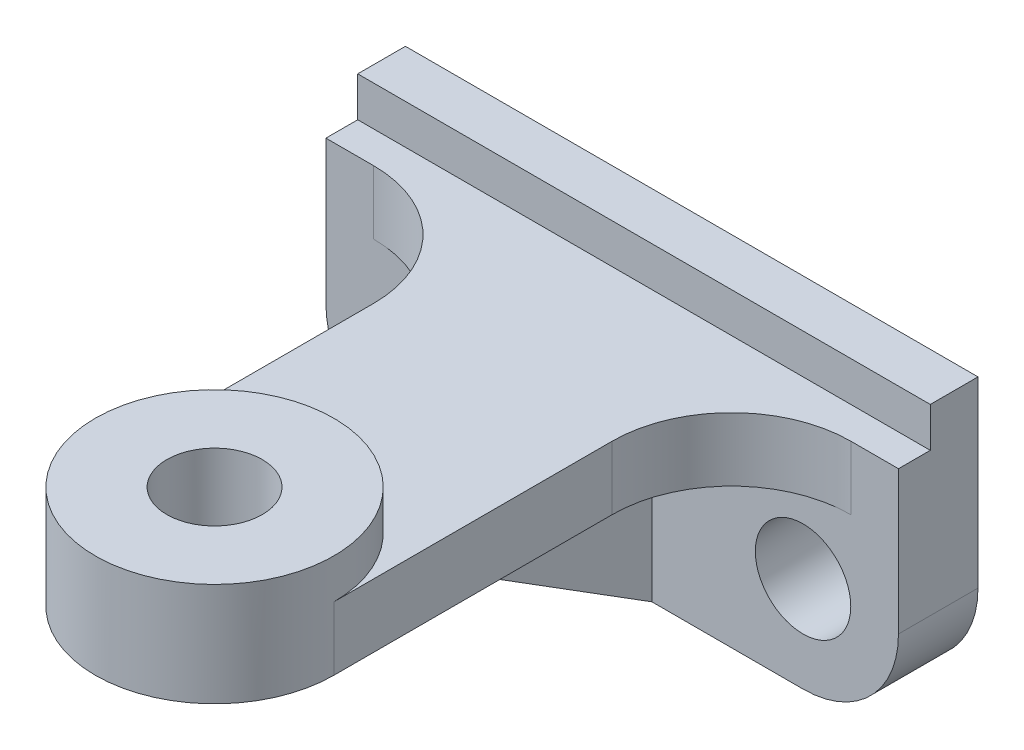
ISO-10303-21;
HEADER;
FILE_DESCRIPTION(('STEP AP214'),'2;1');
FILE_NAME('part.step','',(''),(''),'','','');
FILE_SCHEMA(('AUTOMOTIVE_DESIGN { 1 0 10303 214 1 1 1 1 }'));
ENDSEC;
DATA;
#1=APPLICATION_CONTEXT('core data for automotive mechanical design processes');
#2=APPLICATION_PROTOCOL_DEFINITION('international standard','automotive_design',2000,#1);
#3=PRODUCT_CONTEXT('',#1,'mechanical');
#4=PRODUCT('Part','Part','',(#3));
#5=PRODUCT_RELATED_PRODUCT_CATEGORY('part','',(#4));
#6=PRODUCT_DEFINITION_FORMATION('','',#4);
#7=PRODUCT_DEFINITION_CONTEXT('part definition',#1,'design');
#8=PRODUCT_DEFINITION('design','',#6,#7);
#9=PRODUCT_DEFINITION_SHAPE('','',#8);
#10=(LENGTH_UNIT() NAMED_UNIT(*) SI_UNIT(.MILLI.,.METRE.));
#11=(NAMED_UNIT(*) PLANE_ANGLE_UNIT() SI_UNIT($,.RADIAN.));
#12=(NAMED_UNIT(*) SI_UNIT($,.STERADIAN.) SOLID_ANGLE_UNIT());
#13=UNCERTAINTY_MEASURE_WITH_UNIT(LENGTH_MEASURE(1.E-05),#10,'distance_accuracy_value','');
#14=(GEOMETRIC_REPRESENTATION_CONTEXT(3) GLOBAL_UNCERTAINTY_ASSIGNED_CONTEXT((#13)) GLOBAL_UNIT_ASSIGNED_CONTEXT((#10,
#11,#12)) REPRESENTATION_CONTEXT('',''));
#15=CARTESIAN_POINT('',(0.,0.,0.));
#16=DIRECTION('',(0.,0.,1.));
#17=DIRECTION('',(1.,0.,0.));
#18=AXIS2_PLACEMENT_3D('',#15,#16,#17);
#19=CARTESIAN_POINT('',(72.,-13.,45.0717511200109));
#20=DIRECTION('',(0.,-0.847127010038503,0.531390467418476));
#21=DIRECTION('',(0.,-0.531390467418476,-0.847127010038503));
#22=AXIS2_PLACEMENT_3D('',#19,#20,#21);
#23=PLANE('',#22);
#24=DIRECTION('',(0.,0.531390467418476,0.847127010038503));
#25=VECTOR('',#24,1.);
#26=CARTESIAN_POINT('',(31.,-13.,45.0717511200109));
#27=LINE('',#26,#25);
#28=CARTESIAN_POINT('',(31.,-35.,10.));
#29=VERTEX_POINT('',#28);
#30=CARTESIAN_POINT('',(31.,-13.,45.0717511200109));
#31=VERTEX_POINT('',#30);
#32=EDGE_CURVE('E183',#29,#31,#27,.T.);
#33=ORIENTED_EDGE('',*,*,#32,.F.);
#34=DIRECTION('',(1.,0.,0.));
#35=VECTOR('',#34,1.);
#36=CARTESIAN_POINT('',(0.,-35.,10.));
#37=LINE('',#36,#35);
#38=CARTESIAN_POINT('',(41.,-35.,10.));
#39=VERTEX_POINT('',#38);
#40=EDGE_CURVE('E277',#29,#39,#37,.T.);
#41=ORIENTED_EDGE('',*,*,#40,.T.);
#42=DIRECTION('',(0.,-0.531390467418476,-0.847127010038503));
#43=VECTOR('',#42,1.);
#44=CARTESIAN_POINT('',(41.,-35.,10.));
#45=LINE('',#44,#43);
#46=CARTESIAN_POINT('',(41.,-13.,45.0717511200109));
#47=VERTEX_POINT('',#46);
#48=EDGE_CURVE('E192',#47,#39,#45,.T.);
#49=ORIENTED_EDGE('',*,*,#48,.F.);
#50=DIRECTION('',(-1.,0.,0.));
#51=VECTOR('',#50,1.);
#52=CARTESIAN_POINT('',(72.,-13.,45.0717511200109));
#53=LINE('',#52,#51);
#54=EDGE_CURVE('E180',#47,#31,#53,.T.);
#55=ORIENTED_EDGE('',*,*,#54,.T.);
#56=EDGE_LOOP('',(#33,#41,#49,#55));
#57=FACE_BOUND('',#56,.T.);
#58=ADVANCED_FACE('F50',(#57),#23,.T.);
#59=CARTESIAN_POINT('',(0.,0.,10.));
#60=DIRECTION('',(0.,0.,1.));
#61=DIRECTION('',(1.,0.,0.));
#62=AXIS2_PLACEMENT_3D('',#59,#60,#61);
#63=PLANE('',#62);
#64=DIRECTION('',(0.,-1.,0.));
#65=VECTOR('',#64,1.);
#66=CARTESIAN_POINT('',(66.,-5.,10.));
#67=LINE('',#66,#65);
#68=CARTESIAN_POINT('',(66.,-5.,10.));
#69=VERTEX_POINT('',#68);
#70=CARTESIAN_POINT('',(66.,-13.,10.));
#71=VERTEX_POINT('',#70);
#72=EDGE_CURVE('E212',#69,#71,#67,.T.);
#73=ORIENTED_EDGE('',*,*,#72,.T.);
#74=DIRECTION('',(1.,0.,0.));
#75=VECTOR('',#74,1.);
#76=CARTESIAN_POINT('',(41.,-13.0000000000001,10.));
#77=LINE('',#76,#75);
#78=CARTESIAN_POINT('',(41.,-13.0000000000001,10.));
#79=VERTEX_POINT('',#78);
#80=EDGE_CURVE('E200',#79,#71,#77,.T.);
#81=ORIENTED_EDGE('',*,*,#80,.F.);
#82=DIRECTION('',(0.,1.,0.));
#83=VECTOR('',#82,1.);
#84=CARTESIAN_POINT('',(41.,-13.0000000000001,10.));
#85=LINE('',#84,#83);
#86=EDGE_CURVE('E369',#39,#79,#85,.T.);
#87=ORIENTED_EDGE('',*,*,#86,.F.);
#88=DIRECTION('',(1.,0.,0.));
#89=VECTOR('',#88,1.);
#90=CARTESIAN_POINT('',(41.,-35.,10.));
#91=LINE('',#90,#89);
#92=CARTESIAN_POINT('',(60.,-35.,10.));
#93=VERTEX_POINT('',#92);
#94=EDGE_CURVE('E201',#39,#93,#91,.T.);
#95=ORIENTED_EDGE('',*,*,#94,.T.);
#96=CARTESIAN_POINT('',(60.,-23.,10.));
#97=DIRECTION('',(0.,0.,1.));
#98=DIRECTION('',(1.,0.,0.));
#99=AXIS2_PLACEMENT_3D('',#96,#97,#98);
#100=CIRCLE('',#99,12.);
#101=CARTESIAN_POINT('',(72.,-23.,10.));
#102=VERTEX_POINT('',#101);
#103=EDGE_CURVE('E266',#93,#102,#100,.T.);
#104=ORIENTED_EDGE('',*,*,#103,.T.);
#105=DIRECTION('',(0.,-1.,0.));
#106=VECTOR('',#105,1.);
#107=CARTESIAN_POINT('',(72.,0.,10.));
#108=LINE('',#107,#106);
#109=CARTESIAN_POINT('',(72.,-5.,10.));
#110=VERTEX_POINT('',#109);
#111=EDGE_CURVE('E268',#110,#102,#108,.T.);
#112=ORIENTED_EDGE('',*,*,#111,.F.);
#113=DIRECTION('',(1.,0.,0.));
#114=VECTOR('',#113,1.);
#115=CARTESIAN_POINT('',(0.,-5.00000000000004,10.));
#116=LINE('',#115,#114);
#117=EDGE_CURVE('E310',#69,#110,#116,.T.);
#118=ORIENTED_EDGE('',*,*,#117,.F.);
#119=EDGE_LOOP('',(#73,#81,#87,#95,#104,#112,#118));
#120=FACE_BOUND('',#119,.T.);
#121=CARTESIAN_POINT('',(60.,-23.,10.));
#122=DIRECTION('',(0.,0.,-1.));
#123=DIRECTION('',(-1.,0.,0.));
#124=AXIS2_PLACEMENT_3D('',#121,#122,#123);
#125=CIRCLE('',#124,6.);
#126=CARTESIAN_POINT('',(54.,-23.,10.));
#127=VERTEX_POINT('',#126);
#128=EDGE_CURVE('E194',#127,#127,#125,.F.);
#129=ORIENTED_EDGE('',*,*,#128,.F.);
#130=EDGE_LOOP('',(#129));
#131=FACE_BOUND('',#130,.T.);
#132=ADVANCED_FACE('F316',(#120,#131),#63,.T.);
#133=CARTESIAN_POINT('',(51.,-17.,10.));
#134=DIRECTION('',(1.,0.,0.));
#135=DIRECTION('',(0.,1.,0.));
#136=AXIS2_PLACEMENT_3D('',#133,#134,#135);
#137=PLANE('',#136);
#138=DIRECTION('',(0.,0.,1.));
#139=VECTOR('',#138,1.);
#140=CARTESIAN_POINT('',(51.,-13.,10.));
#141=LINE('',#140,#139);
#142=CARTESIAN_POINT('',(51.,-13.,25.));
#143=VERTEX_POINT('',#142);
#144=CARTESIAN_POINT('',(51.,-13.,60.));
#145=VERTEX_POINT('',#144);
#146=EDGE_CURVE('E235',#143,#145,#141,.T.);
#147=ORIENTED_EDGE('',*,*,#146,.F.);
#148=DIRECTION('',(0.,-1.,0.));
#149=VECTOR('',#148,1.);
#150=CARTESIAN_POINT('',(51.,-5.00000000000001,25.));
#151=LINE('',#150,#149);
#152=CARTESIAN_POINT('',(51.,-5.00000000000001,25.));
#153=VERTEX_POINT('',#152);
#154=EDGE_CURVE('E206',#153,#143,#151,.T.);
#155=ORIENTED_EDGE('',*,*,#154,.F.);
#156=DIRECTION('',(0.,0.,-1.));
#157=VECTOR('',#156,1.);
#158=CARTESIAN_POINT('',(51.,-5.00000000000001,10.));
#159=LINE('',#158,#157);
#160=CARTESIAN_POINT('',(51.,-5.00000000000001,60.));
#161=VERTEX_POINT('',#160);
#162=EDGE_CURVE('E245',#161,#153,#159,.T.);
#163=ORIENTED_EDGE('',*,*,#162,.F.);
#164=DIRECTION('',(0.,1.,0.));
#165=VECTOR('',#164,1.);
#166=CARTESIAN_POINT('',(51.,-17.,60.));
#167=LINE('',#166,#165);
#168=EDGE_CURVE('E248',#145,#161,#167,.T.);
#169=ORIENTED_EDGE('',*,*,#168,.F.);
#170=EDGE_LOOP('',(#147,#155,#163,#169));
#171=FACE_BOUND('',#170,.T.);
#172=ADVANCED_FACE('F366',(#171),#137,.T.);
#173=DIRECTION('',(0.,-1.,0.));
#174=VECTOR('',#173,1.);
#175=CARTESIAN_POINT('',(0.,0.,10.));
#176=LINE('',#175,#174);
#177=CARTESIAN_POINT('',(0.,-5.00000000000002,10.));
#178=VERTEX_POINT('',#177);
#179=CARTESIAN_POINT('',(0.,-23.,10.));
#180=VERTEX_POINT('',#179);
#181=EDGE_CURVE('E275',#178,#180,#176,.T.);
#182=ORIENTED_EDGE('',*,*,#181,.T.);
#183=CARTESIAN_POINT('',(12.,-23.,10.));
#184=DIRECTION('',(0.,0.,1.));
#185=DIRECTION('',(1.,0.,0.));
#186=AXIS2_PLACEMENT_3D('',#183,#184,#185);
#187=CIRCLE('',#186,12.);
#188=CARTESIAN_POINT('',(12.,-35.,10.));
#189=VERTEX_POINT('',#188);
#190=EDGE_CURVE('E274',#180,#189,#187,.T.);
#191=ORIENTED_EDGE('',*,*,#190,.T.);
#192=EDGE_CURVE('E280',#189,#29,#37,.T.);
#193=ORIENTED_EDGE('',*,*,#192,.T.);
#194=DIRECTION('',(0.,-1.,0.));
#195=VECTOR('',#194,1.);
#196=CARTESIAN_POINT('',(31.,-35.,10.));
#197=LINE('',#196,#195);
#198=CARTESIAN_POINT('',(31.,-13.,10.));
#199=VERTEX_POINT('',#198);
#200=EDGE_CURVE('E182',#199,#29,#197,.T.);
#201=ORIENTED_EDGE('',*,*,#200,.F.);
#202=DIRECTION('',(-1.,0.,0.));
#203=VECTOR('',#202,1.);
#204=CARTESIAN_POINT('',(31.,-13.,10.));
#205=LINE('',#204,#203);
#206=CARTESIAN_POINT('',(5.99999999999999,-13.,10.));
#207=VERTEX_POINT('',#206);
#208=EDGE_CURVE('E177',#199,#207,#205,.T.);
#209=ORIENTED_EDGE('',*,*,#208,.T.);
#210=DIRECTION('',(0.,-1.,0.));
#211=VECTOR('',#210,1.);
#212=CARTESIAN_POINT('',(5.99999999999998,-5.00000000000004,10.));
#213=LINE('',#212,#211);
#214=CARTESIAN_POINT('',(5.99999999999998,-5.00000000000004,10.));
#215=VERTEX_POINT('',#214);
#216=EDGE_CURVE('E217',#215,#207,#213,.T.);
#217=ORIENTED_EDGE('',*,*,#216,.F.);
#218=EDGE_CURVE('E57',#178,#215,#116,.T.);
#219=ORIENTED_EDGE('',*,*,#218,.F.);
#220=EDGE_LOOP('',(#182,#191,#193,#201,#209,#217,#219));
#221=FACE_BOUND('',#220,.T.);
#222=CARTESIAN_POINT('',(12.,-23.,10.));
#223=DIRECTION('',(0.,0.,-1.));
#224=DIRECTION('',(-1.,0.,0.));
#225=AXIS2_PLACEMENT_3D('',#222,#223,#224);
#226=CIRCLE('',#225,6.);
#227=CARTESIAN_POINT('',(5.99999999999999,-23.,10.));
#228=VERTEX_POINT('',#227);
#229=EDGE_CURVE('E204',#228,#228,#226,.F.);
#230=ORIENTED_EDGE('',*,*,#229,.F.);
#231=EDGE_LOOP('',(#230));
#232=FACE_BOUND('',#231,.T.);
#233=ADVANCED_FACE('F343',(#221,#232),#63,.T.);
#234=CARTESIAN_POINT('',(36.,-17.,60.));
#235=DIRECTION('',(0.,1.,0.));
#236=DIRECTION('',(-1.,0.,0.));
#237=AXIS2_PLACEMENT_3D('',#234,#235,#236);
#238=CYLINDRICAL_SURFACE('',#237,15.);
#239=CARTESIAN_POINT('',(36.,0.,60.));
#240=DIRECTION('',(0.,1.,0.));
#241=DIRECTION('',(-1.,0.,0.));
#242=AXIS2_PLACEMENT_3D('',#239,#240,#241);
#243=CIRCLE('',#242,15.);
#244=CARTESIAN_POINT('',(21.,0.,60.));
#245=VERTEX_POINT('',#244);
#246=EDGE_CURVE('E237',#245,#245,#243,.T.);
#247=ORIENTED_EDGE('',*,*,#246,.F.);
#248=EDGE_LOOP('',(#247));
#249=FACE_BOUND('',#248,.T.);
#250=DIRECTION('',(0.,1.,0.));
#251=VECTOR('',#250,1.);
#252=CARTESIAN_POINT('',(21.,-17.,60.));
#253=LINE('',#252,#251);
#254=CARTESIAN_POINT('',(21.,-13.,60.));
#255=VERTEX_POINT('',#254);
#256=CARTESIAN_POINT('',(21.,-5.00000000000003,60.));
#257=VERTEX_POINT('',#256);
#258=EDGE_CURVE('E249',#255,#257,#253,.T.);
#259=ORIENTED_EDGE('',*,*,#258,.F.);
#260=CARTESIAN_POINT('',(36.,-13.,60.));
#261=DIRECTION('',(0.,-1.,0.));
#262=DIRECTION('',(1.,0.,0.));
#263=AXIS2_PLACEMENT_3D('',#260,#261,#262);
#264=CIRCLE('',#263,15.);
#265=EDGE_CURVE('E234',#145,#255,#264,.T.);
#266=ORIENTED_EDGE('',*,*,#265,.F.);
#267=ORIENTED_EDGE('',*,*,#168,.T.);
#268=CARTESIAN_POINT('',(36.,-5.00000000000002,60.));
#269=DIRECTION('',(0.,1.,0.));
#270=DIRECTION('',(-1.,0.,0.));
#271=AXIS2_PLACEMENT_3D('',#268,#269,#270);
#272=CIRCLE('',#271,15.);
#273=EDGE_CURVE('E238',#161,#257,#272,.T.);
#274=ORIENTED_EDGE('',*,*,#273,.T.);
#275=EDGE_LOOP('',(#259,#266,#267,#274));
#276=FACE_BOUND('',#275,.T.);
#277=ADVANCED_FACE('F359',(#249,#276),#238,.T.);
#278=CARTESIAN_POINT('',(21.,-17.,60.));
#279=DIRECTION('',(-1.,0.,0.));
#280=DIRECTION('',(0.,-1.,0.));
#281=AXIS2_PLACEMENT_3D('',#278,#279,#280);
#282=PLANE('',#281);
#283=DIRECTION('',(0.,-1.,0.));
#284=VECTOR('',#283,1.);
#285=CARTESIAN_POINT('',(21.,-5.00000000000003,25.));
#286=LINE('',#285,#284);
#287=CARTESIAN_POINT('',(21.,-5.00000000000003,25.));
#288=VERTEX_POINT('',#287);
#289=CARTESIAN_POINT('',(21.,-13.,25.));
#290=VERTEX_POINT('',#289);
#291=EDGE_CURVE('E221',#288,#290,#286,.T.);
#292=ORIENTED_EDGE('',*,*,#291,.T.);
#293=DIRECTION('',(0.,0.,-1.));
#294=VECTOR('',#293,1.);
#295=CARTESIAN_POINT('',(21.,-13.,10.));
#296=LINE('',#295,#294);
#297=EDGE_CURVE('E236',#255,#290,#296,.T.);
#298=ORIENTED_EDGE('',*,*,#297,.F.);
#299=ORIENTED_EDGE('',*,*,#258,.T.);
#300=DIRECTION('',(0.,0.,1.));
#301=VECTOR('',#300,1.);
#302=CARTESIAN_POINT('',(21.,-5.00000000000003,60.));
#303=LINE('',#302,#301);
#304=EDGE_CURVE('E250',#288,#257,#303,.T.);
#305=ORIENTED_EDGE('',*,*,#304,.F.);
#306=EDGE_LOOP('',(#292,#298,#299,#305));
#307=FACE_BOUND('',#306,.T.);
#308=ADVANCED_FACE('F355',(#307),#282,.T.);
#309=CARTESIAN_POINT('',(-78.,-5.00000000000009,6.));
#310=DIRECTION('',(0.,-1.,0.));
#311=DIRECTION('',(1.,0.,0.));
#312=AXIS2_PLACEMENT_3D('',#309,#310,#311);
#313=PLANE('',#312);
#314=CARTESIAN_POINT('',(66.,-5.,25.));
#315=DIRECTION('',(0.,1.,0.));
#316=DIRECTION('',(1.,0.,0.));
#317=AXIS2_PLACEMENT_3D('',#314,#315,#316);
#318=CIRCLE('',#317,15.);
#319=EDGE_CURVE('E207',#69,#153,#318,.T.);
#320=ORIENTED_EDGE('',*,*,#319,.F.);
#321=ORIENTED_EDGE('',*,*,#117,.T.);
#322=DIRECTION('',(0.,0.,-1.));
#323=VECTOR('',#322,1.);
#324=CARTESIAN_POINT('',(72.,-5.,6.));
#325=LINE('',#324,#323);
#326=CARTESIAN_POINT('',(72.,-5.,6.));
#327=VERTEX_POINT('',#326);
#328=EDGE_CURVE('E254',#110,#327,#325,.T.);
#329=ORIENTED_EDGE('',*,*,#328,.T.);
#330=DIRECTION('',(1.,0.,0.));
#331=VECTOR('',#330,1.);
#332=CARTESIAN_POINT('',(-78.,-5.00000000000009,6.));
#333=LINE('',#332,#331);
#334=CARTESIAN_POINT('',(0.,-5.00000000000004,6.));
#335=VERTEX_POINT('',#334);
#336=EDGE_CURVE('E256',#335,#327,#333,.T.);
#337=ORIENTED_EDGE('',*,*,#336,.F.);
#338=DIRECTION('',(0.,0.,-1.));
#339=VECTOR('',#338,1.);
#340=CARTESIAN_POINT('',(0.,-5.00000000000004,10.));
#341=LINE('',#340,#339);
#342=EDGE_CURVE('E72',#178,#335,#341,.T.);
#343=ORIENTED_EDGE('',*,*,#342,.F.);
#344=ORIENTED_EDGE('',*,*,#218,.T.);
#345=CARTESIAN_POINT('',(5.99999999999999,-5.00000000000004,25.));
#346=DIRECTION('',(0.,1.,0.));
#347=DIRECTION('',(-1.,0.,0.));
#348=AXIS2_PLACEMENT_3D('',#345,#346,#347);
#349=CIRCLE('',#348,15.);
#350=EDGE_CURVE('E220',#288,#215,#349,.T.);
#351=ORIENTED_EDGE('',*,*,#350,.F.);
#352=ORIENTED_EDGE('',*,*,#304,.T.);
#353=ORIENTED_EDGE('',*,*,#273,.F.);
#354=ORIENTED_EDGE('',*,*,#162,.T.);
#355=EDGE_LOOP('',(#320,#321,#329,#337,#343,#344,#351,#352,#353,#354));
#356=FACE_BOUND('',#355,.T.);
#357=ADVANCED_FACE('F315',(#356),#313,.F.);
#358=CARTESIAN_POINT('',(60.,-23.,10.));
#359=DIRECTION('',(0.,0.,-1.));
#360=DIRECTION('',(-1.,0.,0.));
#361=AXIS2_PLACEMENT_3D('',#358,#359,#360);
#362=CYLINDRICAL_SURFACE('',#361,12.);
#363=CARTESIAN_POINT('',(60.,-23.,0.));
#364=DIRECTION('',(0.,0.,1.));
#365=DIRECTION('',(1.,0.,0.));
#366=AXIS2_PLACEMENT_3D('',#363,#364,#365);
#367=CIRCLE('',#366,12.);
#368=CARTESIAN_POINT('',(60.,-35.,0.));
#369=VERTEX_POINT('',#368);
#370=CARTESIAN_POINT('',(72.,-23.,0.));
#371=VERTEX_POINT('',#370);
#372=EDGE_CURVE('E264',#369,#371,#367,.T.);
#373=ORIENTED_EDGE('',*,*,#372,.T.);
#374=DIRECTION('',(0.,0.,-1.));
#375=VECTOR('',#374,1.);
#376=CARTESIAN_POINT('',(72.,-23.,10.));
#377=LINE('',#376,#375);
#378=EDGE_CURVE('E304',#102,#371,#377,.T.);
#379=ORIENTED_EDGE('',*,*,#378,.F.);
#380=ORIENTED_EDGE('',*,*,#103,.F.);
#381=DIRECTION('',(0.,0.,-1.));
#382=VECTOR('',#381,1.);
#383=CARTESIAN_POINT('',(60.,-35.,10.));
#384=LINE('',#383,#382);
#385=EDGE_CURVE('E276',#93,#369,#384,.T.);
#386=ORIENTED_EDGE('',*,*,#385,.T.);
#387=EDGE_LOOP('',(#373,#379,#380,#386));
#388=FACE_BOUND('',#387,.T.);
#389=ADVANCED_FACE('F47',(#388),#362,.T.);
#390=CARTESIAN_POINT('',(72.,0.,10.));
#391=DIRECTION('',(1.,0.,0.));
#392=DIRECTION('',(0.,1.,0.));
#393=AXIS2_PLACEMENT_3D('',#390,#391,#392);
#394=PLANE('',#393);
#395=ORIENTED_EDGE('',*,*,#111,.T.);
#396=ORIENTED_EDGE('',*,*,#378,.T.);
#397=DIRECTION('',(0.,-1.,0.));
#398=VECTOR('',#397,1.);
#399=CARTESIAN_POINT('',(72.,0.,0.));
#400=LINE('',#399,#398);
#401=CARTESIAN_POINT('',(72.,0.,0.));
#402=VERTEX_POINT('',#401);
#403=EDGE_CURVE('E285',#402,#371,#400,.T.);
#404=ORIENTED_EDGE('',*,*,#403,.F.);
#405=DIRECTION('',(0.,0.,-1.));
#406=VECTOR('',#405,1.);
#407=CARTESIAN_POINT('',(72.,0.,10.));
#408=LINE('',#407,#406);
#409=CARTESIAN_POINT('',(72.,0.,6.));
#410=VERTEX_POINT('',#409);
#411=EDGE_CURVE('E303',#410,#402,#408,.T.);
#412=ORIENTED_EDGE('',*,*,#411,.F.);
#413=DIRECTION('',(0.,1.,0.));
#414=VECTOR('',#413,1.);
#415=CARTESIAN_POINT('',(72.,0.,6.));
#416=LINE('',#415,#414);
#417=EDGE_CURVE('E260',#327,#410,#416,.T.);
#418=ORIENTED_EDGE('',*,*,#417,.F.);
#419=ORIENTED_EDGE('',*,*,#328,.F.);
#420=EDGE_LOOP('',(#395,#396,#404,#412,#418,#419));
#421=FACE_BOUND('',#420,.T.);
#422=ADVANCED_FACE('F320',(#421),#394,.T.);
#423=CARTESIAN_POINT('',(0.,0.,10.));
#424=DIRECTION('',(0.,1.,0.));
#425=DIRECTION('',(0.,0.,1.));
#426=AXIS2_PLACEMENT_3D('',#423,#424,#425);
#427=PLANE('',#426);
#428=DIRECTION('',(1.,0.,0.));
#429=VECTOR('',#428,1.);
#430=CARTESIAN_POINT('',(-78.,0.,6.));
#431=LINE('',#430,#429);
#432=CARTESIAN_POINT('',(0.,0.,6.));
#433=VERTEX_POINT('',#432);
#434=EDGE_CURVE('E258',#433,#410,#431,.T.);
#435=ORIENTED_EDGE('',*,*,#434,.T.);
#436=ORIENTED_EDGE('',*,*,#411,.T.);
#437=DIRECTION('',(1.,0.,0.));
#438=VECTOR('',#437,1.);
#439=CARTESIAN_POINT('',(0.,0.,0.));
#440=LINE('',#439,#438);
#441=CARTESIAN_POINT('',(0.,0.,0.));
#442=VERTEX_POINT('',#441);
#443=EDGE_CURVE('E284',#442,#402,#440,.T.);
#444=ORIENTED_EDGE('',*,*,#443,.F.);
#445=DIRECTION('',(0.,0.,-1.));
#446=VECTOR('',#445,1.);
#447=CARTESIAN_POINT('',(0.,0.,10.));
#448=LINE('',#447,#446);
#449=EDGE_CURVE('E301',#433,#442,#448,.T.);
#450=ORIENTED_EDGE('',*,*,#449,.F.);
#451=EDGE_LOOP('',(#435,#436,#444,#450));
#452=FACE_BOUND('',#451,.T.);
#453=ADVANCED_FACE('F337',(#452),#427,.T.);
#454=CARTESIAN_POINT('',(0.,0.,10.));
#455=DIRECTION('',(1.,0.,0.));
#456=DIRECTION('',(0.,0.,-1.));
#457=AXIS2_PLACEMENT_3D('',#454,#455,#456);
#458=PLANE('',#457);
#459=DIRECTION('',(0.,0.,-1.));
#460=VECTOR('',#459,1.);
#461=CARTESIAN_POINT('',(0.,-23.,10.));
#462=LINE('',#461,#460);
#463=CARTESIAN_POINT('',(0.,-23.,0.));
#464=VERTEX_POINT('',#463);
#465=EDGE_CURVE('E296',#180,#464,#462,.T.);
#466=ORIENTED_EDGE('',*,*,#465,.F.);
#467=ORIENTED_EDGE('',*,*,#181,.F.);
#468=ORIENTED_EDGE('',*,*,#342,.T.);
#469=DIRECTION('',(0.,1.,0.));
#470=VECTOR('',#469,1.);
#471=CARTESIAN_POINT('',(0.,0.,6.));
#472=LINE('',#471,#470);
#473=EDGE_CURVE('E11',#335,#433,#472,.T.);
#474=ORIENTED_EDGE('',*,*,#473,.T.);
#475=ORIENTED_EDGE('',*,*,#449,.T.);
#476=DIRECTION('',(0.,-1.,0.));
#477=VECTOR('',#476,1.);
#478=CARTESIAN_POINT('',(0.,0.,0.));
#479=LINE('',#478,#477);
#480=EDGE_CURVE('E289',#442,#464,#479,.T.);
#481=ORIENTED_EDGE('',*,*,#480,.T.);
#482=EDGE_LOOP('',(#466,#467,#468,#474,#475,#481));
#483=FACE_BOUND('',#482,.T.);
#484=ADVANCED_FACE('F342',(#483),#458,.F.);
#485=CARTESIAN_POINT('',(12.,-23.,10.));
#486=DIRECTION('',(0.,0.,-1.));
#487=DIRECTION('',(-1.,0.,0.));
#488=AXIS2_PLACEMENT_3D('',#485,#486,#487);
#489=CYLINDRICAL_SURFACE('',#488,12.);
#490=CARTESIAN_POINT('',(12.,-23.,0.));
#491=DIRECTION('',(0.,0.,1.));
#492=DIRECTION('',(1.,0.,0.));
#493=AXIS2_PLACEMENT_3D('',#490,#491,#492);
#494=CIRCLE('',#493,12.);
#495=CARTESIAN_POINT('',(12.,-35.,0.));
#496=VERTEX_POINT('',#495);
#497=EDGE_CURVE('E290',#464,#496,#494,.T.);
#498=ORIENTED_EDGE('',*,*,#497,.T.);
#499=DIRECTION('',(0.,0.,-1.));
#500=VECTOR('',#499,1.);
#501=CARTESIAN_POINT('',(12.,-35.,10.));
#502=LINE('',#501,#500);
#503=EDGE_CURVE('E294',#189,#496,#502,.T.);
#504=ORIENTED_EDGE('',*,*,#503,.F.);
#505=ORIENTED_EDGE('',*,*,#190,.F.);
#506=ORIENTED_EDGE('',*,*,#465,.T.);
#507=EDGE_LOOP('',(#498,#504,#505,#506));
#508=FACE_BOUND('',#507,.T.);
#509=ADVANCED_FACE('F385',(#508),#489,.T.);
#510=CARTESIAN_POINT('',(0.,-35.,10.));
#511=DIRECTION('',(0.,1.,0.));
#512=DIRECTION('',(-1.,0.,0.));
#513=AXIS2_PLACEMENT_3D('',#510,#511,#512);
#514=PLANE('',#513);
#515=DIRECTION('',(1.,0.,0.));
#516=VECTOR('',#515,1.);
#517=CARTESIAN_POINT('',(0.,-35.,0.));
#518=LINE('',#517,#516);
#519=EDGE_CURVE('E270',#496,#369,#518,.T.);
#520=ORIENTED_EDGE('',*,*,#519,.T.);
#521=ORIENTED_EDGE('',*,*,#385,.F.);
#522=ORIENTED_EDGE('',*,*,#94,.F.);
#523=ORIENTED_EDGE('',*,*,#40,.F.);
#524=ORIENTED_EDGE('',*,*,#192,.F.);
#525=ORIENTED_EDGE('',*,*,#503,.T.);
#526=EDGE_LOOP('',(#520,#521,#522,#523,#524,#525));
#527=FACE_BOUND('',#526,.T.);
#528=ADVANCED_FACE('F377',(#527),#514,.F.);
#529=CARTESIAN_POINT('',(0.,0.,0.));
#530=DIRECTION('',(0.,0.,1.));
#531=DIRECTION('',(1.,0.,0.));
#532=AXIS2_PLACEMENT_3D('',#529,#530,#531);
#533=PLANE('',#532);
#534=CARTESIAN_POINT('',(12.,-23.,0.));
#535=DIRECTION('',(0.,0.,1.));
#536=DIRECTION('',(1.,0.,0.));
#537=AXIS2_PLACEMENT_3D('',#534,#535,#536);
#538=CIRCLE('',#537,6.);
#539=CARTESIAN_POINT('',(18.,-23.,0.));
#540=VERTEX_POINT('',#539);
#541=EDGE_CURVE('E51',#540,#540,#538,.T.);
#542=ORIENTED_EDGE('',*,*,#541,.T.);
#543=EDGE_LOOP('',(#542));
#544=FACE_BOUND('',#543,.T.);
#545=CARTESIAN_POINT('',(60.,-23.,0.));
#546=DIRECTION('',(0.,0.,1.));
#547=DIRECTION('',(1.,0.,0.));
#548=AXIS2_PLACEMENT_3D('',#545,#546,#547);
#549=CIRCLE('',#548,6.);
#550=CARTESIAN_POINT('',(66.,-23.,0.));
#551=VERTEX_POINT('',#550);
#552=EDGE_CURVE('E195',#551,#551,#549,.T.);
#553=ORIENTED_EDGE('',*,*,#552,.T.);
#554=EDGE_LOOP('',(#553));
#555=FACE_BOUND('',#554,.T.);
#556=ORIENTED_EDGE('',*,*,#372,.F.);
#557=ORIENTED_EDGE('',*,*,#519,.F.);
#558=ORIENTED_EDGE('',*,*,#497,.F.);
#559=ORIENTED_EDGE('',*,*,#480,.F.);
#560=ORIENTED_EDGE('',*,*,#443,.T.);
#561=ORIENTED_EDGE('',*,*,#403,.T.);
#562=EDGE_LOOP('',(#556,#557,#558,#559,#560,#561));
#563=FACE_BOUND('',#562,.T.);
#564=ADVANCED_FACE('F332',(#544,#555,#563),#533,.F.);
#565=CARTESIAN_POINT('',(-78.,0.,6.));
#566=DIRECTION('',(0.,0.,-1.));
#567=DIRECTION('',(-1.,0.,0.));
#568=AXIS2_PLACEMENT_3D('',#565,#566,#567);
#569=PLANE('',#568);
#570=ORIENTED_EDGE('',*,*,#336,.T.);
#571=ORIENTED_EDGE('',*,*,#417,.T.);
#572=ORIENTED_EDGE('',*,*,#434,.F.);
#573=ORIENTED_EDGE('',*,*,#473,.F.);
#574=EDGE_LOOP('',(#570,#571,#572,#573));
#575=FACE_BOUND('',#574,.T.);
#576=ADVANCED_FACE('F336',(#575),#569,.F.);
#577=CARTESIAN_POINT('',(36.,0.,60.));
#578=DIRECTION('',(0.,1.,0.));
#579=DIRECTION('',(-1.,0.,0.));
#580=AXIS2_PLACEMENT_3D('',#577,#578,#579);
#581=PLANE('',#580);
#582=CARTESIAN_POINT('',(36.,0.,60.));
#583=DIRECTION('',(0.,1.,0.));
#584=DIRECTION('',(-1.,0.,0.));
#585=AXIS2_PLACEMENT_3D('',#582,#583,#584);
#586=CIRCLE('',#585,5.99999999999999);
#587=CARTESIAN_POINT('',(30.,0.,60.));
#588=VERTEX_POINT('',#587);
#589=EDGE_CURVE('E230',#588,#588,#586,.T.);
#590=ORIENTED_EDGE('',*,*,#589,.F.);
#591=EDGE_LOOP('',(#590));
#592=FACE_BOUND('',#591,.T.);
#593=ORIENTED_EDGE('',*,*,#246,.T.);
#594=EDGE_LOOP('',(#593));
#595=FACE_BOUND('',#594,.T.);
#596=ADVANCED_FACE('F419',(#592,#595),#581,.T.);
#597=CARTESIAN_POINT('',(36.,-13.,60.));
#598=DIRECTION('',(0.,-1.,0.));
#599=DIRECTION('',(1.,0.,0.));
#600=AXIS2_PLACEMENT_3D('',#597,#598,#599);
#601=PLANE('',#600);
#602=ORIENTED_EDGE('',*,*,#54,.F.);
#603=DIRECTION('',(0.,0.,1.));
#604=VECTOR('',#603,1.);
#605=CARTESIAN_POINT('',(41.,-13.,45.0717511200109));
#606=LINE('',#605,#604);
#607=EDGE_CURVE('E61',#79,#47,#606,.T.);
#608=ORIENTED_EDGE('',*,*,#607,.F.);
#609=ORIENTED_EDGE('',*,*,#80,.T.);
#610=CARTESIAN_POINT('',(66.,-13.,25.));
#611=DIRECTION('',(0.,1.,0.));
#612=DIRECTION('',(1.,0.,0.));
#613=AXIS2_PLACEMENT_3D('',#610,#611,#612);
#614=CIRCLE('',#613,15.);
#615=EDGE_CURVE('E209',#71,#143,#614,.T.);
#616=ORIENTED_EDGE('',*,*,#615,.T.);
#617=ORIENTED_EDGE('',*,*,#146,.T.);
#618=ORIENTED_EDGE('',*,*,#265,.T.);
#619=ORIENTED_EDGE('',*,*,#297,.T.);
#620=CARTESIAN_POINT('',(6.,-13.,25.));
#621=DIRECTION('',(0.,1.,0.));
#622=DIRECTION('',(-1.,0.,0.));
#623=AXIS2_PLACEMENT_3D('',#620,#621,#622);
#624=CIRCLE('',#623,15.);
#625=EDGE_CURVE('E211',#290,#207,#624,.T.);
#626=ORIENTED_EDGE('',*,*,#625,.T.);
#627=ORIENTED_EDGE('',*,*,#208,.F.);
#628=DIRECTION('',(0.,0.,-1.));
#629=VECTOR('',#628,1.);
#630=CARTESIAN_POINT('',(31.,-13.,10.));
#631=LINE('',#630,#629);
#632=EDGE_CURVE('E175',#31,#199,#631,.T.);
#633=ORIENTED_EDGE('',*,*,#632,.F.);
#634=EDGE_LOOP('',(#602,#608,#609,#616,#617,#618,#619,#626,#627,#633));
#635=FACE_BOUND('',#634,.T.);
#636=CARTESIAN_POINT('',(36.,-13.,60.));
#637=DIRECTION('',(0.,-1.,0.));
#638=DIRECTION('',(1.,0.,0.));
#639=AXIS2_PLACEMENT_3D('',#636,#637,#638);
#640=CIRCLE('',#639,5.99999999999999);
#641=CARTESIAN_POINT('',(42.,-13.,60.));
#642=VERTEX_POINT('',#641);
#643=EDGE_CURVE('E223',#642,#642,#640,.T.);
#644=ORIENTED_EDGE('',*,*,#643,.F.);
#645=EDGE_LOOP('',(#644));
#646=FACE_BOUND('',#645,.T.);
#647=ADVANCED_FACE('F172',(#635,#646),#601,.T.);
#648=CARTESIAN_POINT('',(36.,6.99999999999998,60.));
#649=DIRECTION('',(0.,-1.,0.));
#650=DIRECTION('',(1.,0.,0.));
#651=AXIS2_PLACEMENT_3D('',#648,#649,#650);
#652=CYLINDRICAL_SURFACE('',#651,5.99999999999999);
#653=ORIENTED_EDGE('',*,*,#589,.T.);
#654=EDGE_LOOP('',(#653));
#655=FACE_BOUND('',#654,.T.);
#656=ORIENTED_EDGE('',*,*,#643,.T.);
#657=EDGE_LOOP('',(#656));
#658=FACE_BOUND('',#657,.T.);
#659=ADVANCED_FACE('F415',(#655,#658),#652,.F.);
#660=CARTESIAN_POINT('',(5.99999999999999,-5.00000000000004,25.));
#661=DIRECTION('',(0.,-1.,0.));
#662=DIRECTION('',(1.,0.,0.));
#663=AXIS2_PLACEMENT_3D('',#660,#661,#662);
#664=CYLINDRICAL_SURFACE('',#663,15.);
#665=ORIENTED_EDGE('',*,*,#625,.F.);
#666=ORIENTED_EDGE('',*,*,#291,.F.);
#667=ORIENTED_EDGE('',*,*,#350,.T.);
#668=ORIENTED_EDGE('',*,*,#216,.T.);
#669=EDGE_LOOP('',(#665,#666,#667,#668));
#670=FACE_BOUND('',#669,.T.);
#671=ADVANCED_FACE('F351',(#670),#664,.F.);
#672=CARTESIAN_POINT('',(66.,-5.,25.));
#673=DIRECTION('',(0.,-1.,0.));
#674=DIRECTION('',(1.,0.,0.));
#675=AXIS2_PLACEMENT_3D('',#672,#673,#674);
#676=CYLINDRICAL_SURFACE('',#675,15.);
#677=ORIENTED_EDGE('',*,*,#615,.F.);
#678=ORIENTED_EDGE('',*,*,#72,.F.);
#679=ORIENTED_EDGE('',*,*,#319,.T.);
#680=ORIENTED_EDGE('',*,*,#154,.T.);
#681=EDGE_LOOP('',(#677,#678,#679,#680));
#682=FACE_BOUND('',#681,.T.);
#683=ADVANCED_FACE('F367',(#682),#676,.F.);
#684=CARTESIAN_POINT('',(60.,-23.,-10.));
#685=DIRECTION('',(0.,0.,1.));
#686=DIRECTION('',(1.,0.,0.));
#687=AXIS2_PLACEMENT_3D('',#684,#685,#686);
#688=CYLINDRICAL_SURFACE('',#687,6.);
#689=ORIENTED_EDGE('',*,*,#128,.T.);
#690=EDGE_LOOP('',(#689));
#691=FACE_BOUND('',#690,.T.);
#692=ORIENTED_EDGE('',*,*,#552,.F.);
#693=EDGE_LOOP('',(#692));
#694=FACE_BOUND('',#693,.T.);
#695=ADVANCED_FACE('F401',(#691,#694),#688,.F.);
#696=CARTESIAN_POINT('',(12.,-23.,-10.));
#697=DIRECTION('',(0.,0.,1.));
#698=DIRECTION('',(1.,0.,0.));
#699=AXIS2_PLACEMENT_3D('',#696,#697,#698);
#700=CYLINDRICAL_SURFACE('',#699,6.);
#701=ORIENTED_EDGE('',*,*,#229,.T.);
#702=EDGE_LOOP('',(#701));
#703=FACE_BOUND('',#702,.T.);
#704=ORIENTED_EDGE('',*,*,#541,.F.);
#705=EDGE_LOOP('',(#704));
#706=FACE_BOUND('',#705,.T.);
#707=ADVANCED_FACE('F400',(#703,#706),#700,.F.);
#708=CARTESIAN_POINT('',(41.,0.,0.));
#709=DIRECTION('',(1.,0.,0.));
#710=DIRECTION('',(0.,1.,0.));
#711=AXIS2_PLACEMENT_3D('',#708,#709,#710);
#712=PLANE('',#711);
#713=ORIENTED_EDGE('',*,*,#48,.T.);
#714=ORIENTED_EDGE('',*,*,#86,.T.);
#715=ORIENTED_EDGE('',*,*,#607,.T.);
#716=EDGE_LOOP('',(#713,#714,#715));
#717=FACE_BOUND('',#716,.T.);
#718=ADVANCED_FACE('F371',(#717),#712,.T.);
#719=CARTESIAN_POINT('',(31.,0.,0.));
#720=DIRECTION('',(1.,0.,0.));
#721=DIRECTION('',(0.,0.,-1.));
#722=AXIS2_PLACEMENT_3D('',#719,#720,#721);
#723=PLANE('',#722);
#724=ORIENTED_EDGE('',*,*,#32,.T.);
#725=ORIENTED_EDGE('',*,*,#632,.T.);
#726=ORIENTED_EDGE('',*,*,#200,.T.);
#727=EDGE_LOOP('',(#724,#725,#726));
#728=FACE_BOUND('',#727,.T.);
#729=ADVANCED_FACE('F190',(#728),#723,.F.);
#730=CLOSED_SHELL('',(#58,#132,#172,#233,#277,#308,#357,#389,#422,#453,#484,#509,#528,#564,#576,
#596,#647,#659,#671,#683,#695,#707,#718,#729));
#731=MANIFOLD_SOLID_BREP('B2',#730);
#732=ADVANCED_BREP_SHAPE_REPRESENTATION('',(#18,#731),#14);
#733=SHAPE_DEFINITION_REPRESENTATION(#9,#732);
ENDSEC;
END-ISO-10303-21;
